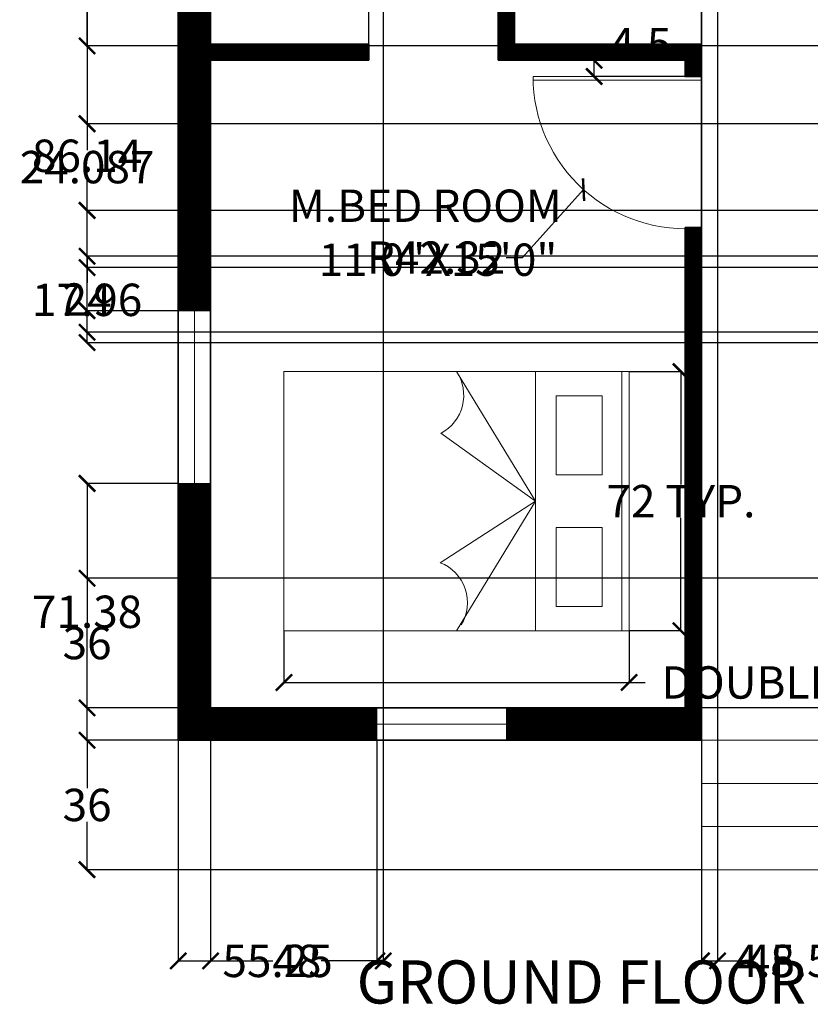
# Model space of a CAD drawing. Units: inches. Extents: x -1 to 426, y -6 to 532.
# Tile 1 of 4: x -1 to 219, y -6 to 267. Entities that reach past the tile are written whole.
import ezdxf

# ---------------------------------------------------------------- set-up
doc = ezdxf.new("R2010")
doc.units = ezdxf.units.IN
doc.header["$MEASUREMENT"] = 0
for name, color, linetype, lineweight in [('A-ANNO-DIMS', 2, 'Continuous', 18), ('A-ANNO-TEXT', 7, 'Continuous', 35), ('A-AREA-IDEN', 7, 'Continuous', 25), ('A-DOOR', 3, 'Continuous', 18), ('A-FLOR-STRS', 42, 'Continuous', 18), ('A-FURN', 8, 'Continuous', 18), ('A-GLAZ', 4, 'Continuous', 18)]:
    doc.layers.add(name, color=color, linetype=linetype, lineweight=lineweight)
doc.layers.add('A-WALL', color=159, linetype='Continuous', lineweight=35, true_color=0x223569)
doc.layers.add('A-WALL-PATT', color=177, linetype='Continuous', lineweight=13, true_color=0x2c4178)
doc.styles.get("Standard").update_dxf_attribs({"font": 'arial.ttf'})
doc.dimstyles.get("Standard").update_dxf_attribs({"dimtxt": 9, "dimasz": 4.5, "dimexe": 0.18, "dimexo": 0.0625, "dimgap": 0.09, "dimtad": 0, "dimtih": 1, "dimtoh": 1, "dimdec": 1, "dimzin": 0, "dimdsep": 46, "dimlunit": 4, "dimtxsty": 'Standard', "dimblk": 'ARCHTICK', "dimcen": 0.09, "dimadec": 0, "dimazin": 0, "dimtfac": 1, "dimtdec": 1, "dimtofl": 0, "dimtmove": 0, "dimatfit": 3, "dimfxl": 1, "dimtolj": 1, "dimtzin": 0, "dimarcsym": 0})

# ---------------------------------------------------------------- blocks, each defined once
blk = doc.blocks.new('WIN-36IN')
for p, q in [((0, 4.5), (36, 4.5)), ((0, -4.5), (0, 4.5)), ((36, 4.5), (36, -4.5)), ((0, 0), (36, 0)), ((36, -4.5), (0, -4.5))]:
    blk.add_line(p, q)
blk = doc.blocks.new('WIN-48IN')
for p, q in [((-4.5, 48), (4.5, 48)), ((-4.5, 0), (-4.5, 48)), ((0, 48), (0, 0)), ((4.5, 48), (4.5, 0)), ((4.5, 0), (-4.5, 0))]:
    blk.add_line(p, q)
blk = doc.blocks.new('BED-DOUBLE')
for p, q in [((-96, 0), (-96, 72)), ((-96, 72), (0, 72)), ((-26, 36), (-48, 72)), ((-26, 72), (-26, 0)), ((-2, 72), (-2, 0)), ((0, 72), (0, 0)), ((-52.33, 54.93), (-26, 36)), ((-26, 36), (-52.6, 18.9)), ((-48, 0), (-26, 36)), ((0, 0), (-96, 0))]:
    blk.add_line(p, q)
for points in [[(-7.5, 65.27), (-7.5, 43.28), (-20.33, 43.28), (-20.33, 65.27)], [(-7.5, 6.73), (-7.5, 28.72), (-20.33, 28.72), (-20.33, 6.73)]]:
    blk.add_lwpolyline(points, close=True)
for centre, start, end in [((-57.86, 65.42), 297.83, 33.7219), ((-56.81, 7.81), 328.371, 69.2037)]:
    blk.add_arc(centre, 11.86, start, end)
blk = doc.blocks.new('_ArchTick')
at = {"color": 0, "linetype": 'ByBlock', "const_width": 0.15}
blk.add_lwpolyline([(-0.5, -0.5), (0.5, 0.5)], dxfattribs=at)
blk = doc.blocks.new('*D11')
at = {"layer": 'A-ANNO-DIMS', "color": 0, "lineweight": -2, "transparency": 16777216}
for p, q in [((72.72, 97.36), (72.72, 82.85)), ((168.72, 97.36), (168.72, 82.85)), ((72.72, 83.03), (168.72, 83.03)), ((168.72, 83.03), (173.22, 83.03))]:
    blk.add_line(p, q, dxfattribs=at)
at = {"layer": 'Defpoints', "color": 0, "transparency": 16777216}
for p in [(72.72, 97.43), (168.72, 97.43), (168.72, 83.03)]:
    blk.add_point(p, dxfattribs=at)
at = {"layer": 'A-ANNO-DIMS', "color": 0, "lineweight": -2, "transparency": 16777216, "xscale": 4.5, "yscale": 4.5, "zscale": 4.5, "rotation": 180}
blk.add_blockref('_ArchTick', (72.72, 83.03), dxfattribs=at)
at = {"layer": 'A-ANNO-DIMS', "color": 0, "lineweight": -2, "transparency": 16777216, "xscale": 4.5, "yscale": 4.5, "zscale": 4.5}
blk.add_blockref('_ArchTick', (168.72, 83.03), dxfattribs=at)
at = {"layer": 'A-ANNO-DIMS', "color": 0, "transparency": 16777216, "insert": (237.26, 83.03), "char_height": 9, "attachment_point": 5}
blk.add_mtext('\\A1;DOUBLE BED 96 TYP.', dxfattribs=at)
blk = doc.blocks.new('*D12')
at = {"layer": 'A-ANNO-DIMS', "color": 0, "lineweight": -2, "transparency": 16777216}
for p, q in [((168.78, 169.43), (183.3, 169.43)), ((183.12, 169.43), (183.12, 138.04)), ((183.12, 97.43), (183.12, 128.81)), ((168.78, 97.43), (183.3, 97.43))]:
    blk.add_line(p, q, dxfattribs=at)
at = {"layer": 'Defpoints', "color": 0, "transparency": 16777216}
for p in [(168.72, 169.43), (183.12, 169.43), (168.72, 97.43)]:
    blk.add_point(p, dxfattribs=at)
at = {"layer": 'A-ANNO-DIMS', "color": 0, "lineweight": -2, "transparency": 16777216, "xscale": 4.5, "yscale": 4.5, "zscale": 4.5}
for p, rotation in [((183.12, 169.43), 90), ((183.12, 97.43), 270)]:
    blk.add_blockref('_ArchTick', p, dxfattribs=dict(at, rotation=rotation))
at = {"layer": 'A-ANNO-DIMS', "color": 0, "transparency": 16777216, "insert": (183.12, 133.43), "char_height": 9, "attachment_point": 5}
blk.add_mtext('\\A1;72 TYP.', dxfattribs=at)
blk = doc.blocks.new('*D19')
at = {"layer": 'A-ANNO-DIMS', "color": 0, "lineweight": -2, "transparency": 16777216}
for p, q in [((188.76, 66.98), (17.79, 66.98)), ((17.97, 66.98), (17.97, 53.67)), ((17.97, 30.98), (17.97, 44.29)), ((188.76, 30.98), (17.79, 30.98))]:
    blk.add_line(p, q, dxfattribs=at)
at = {"layer": 'Defpoints', "color": 0, "transparency": 16777216}
for p in [(17.97, 66.98), (188.82, 66.98), (188.82, 30.98)]:
    blk.add_point(p, dxfattribs=at)
at = {"layer": 'A-ANNO-DIMS', "color": 0, "lineweight": -2, "transparency": 16777216, "xscale": 4.5, "yscale": 4.5, "zscale": 4.5}
for p, rotation in [((17.97, 66.98), 90), ((17.97, 30.98), 270)]:
    blk.add_blockref('_ArchTick', p, dxfattribs=dict(at, rotation=rotation))
at = {"layer": 'A-ANNO-DIMS', "color": 0, "transparency": 16777216, "insert": (17.97, 48.98), "char_height": 9, "attachment_point": 5}
blk.add_mtext('\\A1;36', dxfattribs=at)
blk = doc.blocks.new('*D20')
at = {"layer": 'A-ANNO-DIMS', "color": 0, "lineweight": -2, "transparency": 16777216}
for p, q in [((43.32, 67.04), (43.32, 526.02)), ((43.32, 525.84), (101.19, 525.84)), ((188.82, 525.84), (130.96, 525.84)), ((188.82, 67.04), (188.82, 526.02))]:
    blk.add_line(p, q, dxfattribs=at)
at = {"layer": 'Defpoints', "color": 0, "transparency": 16777216}
for p in [(188.82, 525.84), (43.32, 66.98), (188.82, 66.98)]:
    blk.add_point(p, dxfattribs=at)
at = {"layer": 'A-ANNO-DIMS', "color": 0, "lineweight": -2, "transparency": 16777216, "xscale": 4.5, "yscale": 4.5, "zscale": 4.5, "rotation": 180}
blk.add_blockref('_ArchTick', (43.32, 525.84), dxfattribs=at)
at = {"layer": 'A-ANNO-DIMS', "color": 0, "lineweight": -2, "transparency": 16777216, "xscale": 4.5, "yscale": 4.5, "zscale": 4.5}
blk.add_blockref('_ArchTick', (188.82, 525.84), dxfattribs=at)
at = {"layer": 'A-ANNO-DIMS', "color": 0, "transparency": 16777216, "insert": (116.07, 525.84), "char_height": 9, "attachment_point": 5}
blk.add_mtext('\\A1;145.5', dxfattribs=at)
blk = doc.blocks.new('*D21')
at = {"layer": 'A-ANNO-DIMS', "color": 0, "lineweight": -2, "transparency": 16777216}
for p, q in [((188.82, 30.92), (188.82, 5.45)), ((237.32, 30.92), (237.32, 5.45)), ((188.82, 5.63), (201.08, 5.63)), ((237.32, 5.63), (225.07, 5.63))]:
    blk.add_line(p, q, dxfattribs=at)
at = {"layer": 'Defpoints', "color": 0, "transparency": 16777216}
for p in [(188.82, 30.98), (237.32, 30.98), (237.32, 5.63)]:
    blk.add_point(p, dxfattribs=at)
at = {"layer": 'A-ANNO-DIMS', "color": 0, "lineweight": -2, "transparency": 16777216, "xscale": 4.5, "yscale": 4.5, "zscale": 4.5, "rotation": 180}
blk.add_blockref('_ArchTick', (188.82, 5.63), dxfattribs=at)
at = {"layer": 'A-ANNO-DIMS', "color": 0, "lineweight": -2, "transparency": 16777216, "xscale": 4.5, "yscale": 4.5, "zscale": 4.5}
blk.add_blockref('_ArchTick', (237.32, 5.63), dxfattribs=at)
at = {"layer": 'A-ANNO-DIMS', "color": 0, "transparency": 16777216, "insert": (213.07, 5.63), "char_height": 9, "attachment_point": 5}
blk.add_mtext('\\A1;48.5', dxfattribs=at)
blk = doc.blocks.new('*D22')
at = {"layer": 'A-ANNO-DIMS', "color": 0, "lineweight": -2, "transparency": 16777216}
for p, q in [((52.32, 491.42), (52.32, 5.45)), ((100.32, 491.42), (100.32, 5.45)), ((52.32, 5.63), (69.6, 5.63)), ((100.32, 5.63), (83.05, 5.63))]:
    blk.add_line(p, q, dxfattribs=at)
at = {"layer": 'Defpoints', "color": 0, "transparency": 16777216}
for p in [(52.32, 491.48), (100.32, 491.48), (100.32, 5.63)]:
    blk.add_point(p, dxfattribs=at)
at = {"layer": 'A-ANNO-DIMS', "color": 0, "lineweight": -2, "transparency": 16777216, "xscale": 4.5, "yscale": 4.5, "zscale": 4.5, "rotation": 180}
blk.add_blockref('_ArchTick', (52.32, 5.63), dxfattribs=at)
at = {"layer": 'A-ANNO-DIMS', "color": 0, "lineweight": -2, "transparency": 16777216, "xscale": 4.5, "yscale": 4.5, "zscale": 4.5}
blk.add_blockref('_ArchTick', (100.32, 5.63), dxfattribs=at)
at = {"layer": 'A-ANNO-DIMS', "color": 0, "transparency": 16777216, "insert": (76.32, 5.63), "char_height": 9, "attachment_point": 5}
blk.add_mtext('\\A1;48', dxfattribs=at)
blk = doc.blocks.new('*D24')
at = {"layer": 'A-ANNO-DIMS', "color": 0, "lineweight": -2, "transparency": 16777216}
for p, q in [((43.32, 66.92), (43.32, 5.45)), ((98.58, 66.92), (98.58, 5.45)), ((43.32, 5.63), (55.64, 5.63)), ((98.58, 5.63), (86.26, 5.63))]:
    blk.add_line(p, q, dxfattribs=at)
at = {"layer": 'Defpoints', "color": 0, "transparency": 16777216}
for p in [(43.32, 66.98), (98.58, 66.98), (98.58, 5.63)]:
    blk.add_point(p, dxfattribs=at)
at = {"layer": 'A-ANNO-DIMS', "color": 0, "lineweight": -2, "transparency": 16777216, "xscale": 4.5, "yscale": 4.5, "zscale": 4.5, "rotation": 180}
blk.add_blockref('_ArchTick', (43.32, 5.63), dxfattribs=at)
at = {"layer": 'A-ANNO-DIMS', "color": 0, "lineweight": -2, "transparency": 16777216, "xscale": 4.5, "yscale": 4.5, "zscale": 4.5}
blk.add_blockref('_ArchTick', (98.58, 5.63), dxfattribs=at)
at = {"layer": 'A-ANNO-DIMS', "color": 0, "transparency": 16777216, "insert": (70.95, 5.63), "char_height": 9, "attachment_point": 5}
blk.add_mtext('\\A1;55.25', dxfattribs=at)
blk = doc.blocks.new('*D25')
at = {"layer": 'A-ANNO-DIMS', "color": 0, "lineweight": -2, "transparency": 16777216}
for p, q in [((43.26, 138.36), (17.79, 138.36)), ((17.97, 138.36), (17.97, 107.36)), ((17.97, 66.98), (17.97, 97.98)), ((43.26, 66.98), (17.79, 66.98))]:
    blk.add_line(p, q, dxfattribs=at)
at = {"layer": 'Defpoints', "color": 0, "transparency": 16777216}
for p in [(17.97, 138.36), (43.32, 138.36), (43.32, 66.98)]:
    blk.add_point(p, dxfattribs=at)
at = {"layer": 'A-ANNO-DIMS', "color": 0, "lineweight": -2, "transparency": 16777216, "xscale": 4.5, "yscale": 4.5, "zscale": 4.5}
for p, rotation in [((17.97, 138.36), 90), ((17.97, 66.98), 270)]:
    blk.add_blockref('_ArchTick', p, dxfattribs=dict(at, rotation=rotation))
at = {"layer": 'A-ANNO-DIMS', "color": 0, "transparency": 16777216, "insert": (17.97, 102.67), "char_height": 9, "attachment_point": 5}
blk.add_mtext('\\A1;71.38', dxfattribs=at)
blk = doc.blocks.new('*D26')
at = {"layer": 'A-ANNO-DIMS', "color": 0, "lineweight": -2, "transparency": 16777216}
for p, q in [((43.26, 272.5), (17.79, 272.5)), ((17.97, 272.5), (17.97, 234.11)), ((17.97, 186.36), (17.97, 224.74)), ((43.26, 186.36), (17.79, 186.36))]:
    blk.add_line(p, q, dxfattribs=at)
at = {"layer": 'Defpoints', "color": 0, "transparency": 16777216}
for p in [(17.97, 272.5), (43.32, 272.5), (43.32, 186.36)]:
    blk.add_point(p, dxfattribs=at)
at = {"layer": 'A-ANNO-DIMS', "color": 0, "lineweight": -2, "transparency": 16777216, "xscale": 4.5, "yscale": 4.5, "zscale": 4.5}
for p, rotation in [((17.97, 272.5), 90), ((17.97, 186.36), 270)]:
    blk.add_blockref('_ArchTick', p, dxfattribs=dict(at, rotation=rotation))
at = {"layer": 'A-ANNO-DIMS', "color": 0, "transparency": 16777216, "insert": (17.97, 229.43), "char_height": 9, "attachment_point": 5}
blk.add_mtext('\\A1;86.14', dxfattribs=at)
blk = doc.blocks.new('*D32')
at = {"layer": 'A-ANNO-DIMS', "color": 0, "lineweight": -2, "transparency": 16777216}
for p, q in [((331.76, 293.06), (17.79, 293.06)), ((17.97, 293.06), (17.97, 281.21)), ((17.97, 259.98), (17.97, 271.83)), ((331.76, 259.98), (17.79, 259.98))]:
    blk.add_line(p, q, dxfattribs=at)
at = {"layer": 'Defpoints', "color": 0, "transparency": 16777216}
for p in [(17.97, 293.06), (331.82, 293.06), (331.82, 259.98)]:
    blk.add_point(p, dxfattribs=at)
at = {"layer": 'A-ANNO-DIMS', "color": 0, "lineweight": -2, "transparency": 16777216, "xscale": 4.5, "yscale": 4.5, "zscale": 4.5}
for p, rotation in [((17.97, 293.06), 90), ((17.97, 259.98), 270)]:
    blk.add_blockref('_ArchTick', p, dxfattribs=dict(at, rotation=rotation))
at = {"layer": 'A-ANNO-DIMS', "color": 0, "transparency": 16777216, "insert": (17.97, 276.52), "char_height": 9, "attachment_point": 5}
blk.add_mtext('\\A1;33.08', dxfattribs=at)
blk = doc.blocks.new('*D34')
at = {"layer": 'A-ANNO-DIMS', "color": 0, "lineweight": -2, "transparency": 16777216}
for p, q in [((237.26, 111.98), (17.79, 111.98)), ((17.97, 111.98), (17.97, 98.67)), ((17.97, 75.98), (17.97, 89.29)), ((237.26, 75.98), (17.79, 75.98))]:
    blk.add_line(p, q, dxfattribs=at)
at = {"layer": 'Defpoints', "color": 0, "transparency": 16777216}
for p in [(17.97, 111.98), (237.32, 111.98), (237.32, 75.98)]:
    blk.add_point(p, dxfattribs=at)
at = {"layer": 'A-ANNO-DIMS', "color": 0, "lineweight": -2, "transparency": 16777216, "xscale": 4.5, "yscale": 4.5, "zscale": 4.5}
for p, rotation in [((17.97, 111.98), 90), ((17.97, 75.98), 270)]:
    blk.add_blockref('_ArchTick', p, dxfattribs=dict(at, rotation=rotation))
at = {"layer": 'A-ANNO-DIMS', "color": 0, "transparency": 16777216, "insert": (17.97, 93.98), "char_height": 9, "attachment_point": 5}
blk.add_mtext('\\A1;36', dxfattribs=at)
blk = doc.blocks.new('*D37')
at = {"layer": 'A-ANNO-DIMS', "color": 0, "lineweight": -2, "transparency": 16777216}
for p, q in [((258.34, 198.36), (17.79, 198.36)), ((17.97, 198.36), (17.97, 194.07)), ((17.97, 180.4), (17.97, 184.7)), ((258.34, 180.4), (17.79, 180.4))]:
    blk.add_line(p, q, dxfattribs=at)
at = {"layer": 'Defpoints', "color": 0, "transparency": 16777216}
for p in [(17.97, 198.36), (258.4, 198.36), (258.4, 180.4)]:
    blk.add_point(p, dxfattribs=at)
at = {"layer": 'A-ANNO-DIMS', "color": 0, "lineweight": -2, "transparency": 16777216, "xscale": 4.5, "yscale": 4.5, "zscale": 4.5}
for p, rotation in [((17.97, 198.36), 90), ((17.97, 180.4), 270)]:
    blk.add_blockref('_ArchTick', p, dxfattribs=dict(at, rotation=rotation))
at = {"layer": 'A-ANNO-DIMS', "color": 0, "transparency": 16777216, "insert": (17.97, 189.38), "char_height": 9, "attachment_point": 5}
blk.add_mtext('\\A1;17.96', dxfattribs=at)
blk = doc.blocks.new('*D39')
at = {"layer": 'A-ANNO-DIMS', "color": 0, "lineweight": -2, "transparency": 16777216}
for p, q in [((96.36, 256.04), (96.36, 526.02)), ((96.36, 525.84), (132.32, 525.84)), ((132.32, 256.04), (132.32, 526.02)), ((132.32, 525.84), (136.82, 525.84))]:
    blk.add_line(p, q, dxfattribs=at)
at = {"layer": 'Defpoints', "color": 0, "transparency": 16777216}
for p in [(132.32, 525.84), (96.36, 255.98), (132.32, 255.98)]:
    blk.add_point(p, dxfattribs=at)
at = {"layer": 'A-ANNO-DIMS', "color": 0, "lineweight": -2, "transparency": 16777216, "xscale": 4.5, "yscale": 4.5, "zscale": 4.5, "rotation": 180}
blk.add_blockref('_ArchTick', (96.36, 525.84), dxfattribs=at)
at = {"layer": 'A-ANNO-DIMS', "color": 0, "lineweight": -2, "transparency": 16777216, "xscale": 4.5, "yscale": 4.5, "zscale": 4.5}
blk.add_blockref('_ArchTick', (132.32, 525.84), dxfattribs=at)
at = {"layer": 'A-ANNO-DIMS', "color": 0, "transparency": 16777216, "insert": (155.63, 525.84), "char_height": 9, "attachment_point": 5}
blk.add_mtext('\\A1;35.965', dxfattribs=at)
blk = doc.blocks.new('*D45')
at = {"layer": 'A-ANNO-DIMS', "color": 0, "lineweight": -2, "transparency": 16777216}
for p, q in [((241.76, 201.48), (17.79, 201.48)), ((17.97, 201.48), (17.97, 194.09)), ((17.97, 177.48), (17.97, 184.87)), ((241.76, 177.48), (17.79, 177.48))]:
    blk.add_line(p, q, dxfattribs=at)
at = {"layer": 'Defpoints', "color": 0, "transparency": 16777216}
for p in [(17.97, 201.48), (241.82, 201.48), (241.82, 177.48)]:
    blk.add_point(p, dxfattribs=at)
at = {"layer": 'A-ANNO-DIMS', "color": 0, "lineweight": -2, "transparency": 16777216, "xscale": 4.5, "yscale": 4.5, "zscale": 4.5}
for p, rotation in [((17.97, 201.48), 90), ((17.97, 177.48), 270)]:
    blk.add_blockref('_ArchTick', p, dxfattribs=dict(at, rotation=rotation))
at = {"layer": 'A-ANNO-DIMS', "color": 0, "transparency": 16777216, "insert": (17.97, 189.48), "char_height": 9, "attachment_point": 5}
blk.add_mtext('\\A1;24', dxfattribs=at)
blk = doc.blocks.new('*D47')
at = {"layer": 'A-ANNO-DIMS', "color": 0, "lineweight": -2, "transparency": 16777216}
for p, q in [((188.82, 412.42), (188.82, 5.45)), ((193.32, 412.42), (193.32, 5.45)), ((188.82, 5.63), (193.32, 5.63)), ((193.32, 5.63), (197.82, 5.63))]:
    blk.add_line(p, q, dxfattribs=at)
at = {"layer": 'Defpoints', "color": 0, "transparency": 16777216}
for p in [(188.82, 412.48), (193.32, 412.48), (193.32, 5.63)]:
    blk.add_point(p, dxfattribs=at)
at = {"layer": 'A-ANNO-DIMS', "color": 0, "lineweight": -2, "transparency": 16777216, "xscale": 4.5, "yscale": 4.5, "zscale": 4.5, "rotation": 180}
blk.add_blockref('_ArchTick', (188.82, 5.63), dxfattribs=at)
at = {"layer": 'A-ANNO-DIMS', "color": 0, "lineweight": -2, "transparency": 16777216, "xscale": 4.5, "yscale": 4.5, "zscale": 4.5}
blk.add_blockref('_ArchTick', (193.32, 5.63), dxfattribs=at)
at = {"layer": 'A-ANNO-DIMS', "color": 0, "transparency": 16777216, "insert": (206.32, 5.63), "char_height": 9, "attachment_point": 5}
blk.add_mtext('\\A1;4.5', dxfattribs=at)
blk = doc.blocks.new('*D51')
at = {"layer": 'A-ANNO-DIMS', "color": 0, "lineweight": -2, "transparency": 16777216}
for p, q in [((158.97, 255.98), (158.97, 260.48)), ((158.97, 260.48), (163.47, 260.48)), ((184.26, 255.98), (158.79, 255.98)), ((158.97, 251.48), (158.97, 255.98)), ((184.26, 251.48), (158.79, 251.48))]:
    blk.add_line(p, q, dxfattribs=at)
at = {"layer": 'Defpoints', "color": 0, "transparency": 16777216}
for p in [(158.97, 255.98), (184.32, 255.98), (184.32, 251.48)]:
    blk.add_point(p, dxfattribs=at)
at = {"layer": 'A-ANNO-DIMS', "color": 0, "lineweight": -2, "transparency": 16777216, "xscale": 4.5, "yscale": 4.5, "zscale": 4.5}
for p, rotation in [((158.97, 255.98), 90), ((158.97, 251.48), 270)]:
    blk.add_blockref('_ArchTick', p, dxfattribs=dict(at, rotation=rotation))
at = {"layer": 'A-ANNO-DIMS', "color": 0, "transparency": 16777216, "insert": (171.96, 260.48), "char_height": 9, "attachment_point": 5}
blk.add_mtext('\\A1;4.5', dxfattribs=at)
blk = doc.blocks.new('*D53')
at = {"layer": 'A-ANNO-DIMS', "color": 0, "lineweight": -2, "transparency": 16777216}
for p, q in [((313, 238.33), (17.79, 238.33)), ((17.97, 238.33), (17.97, 230.97)), ((17.97, 214.24), (17.97, 221.6)), ((313, 214.24), (17.79, 214.24))]:
    blk.add_line(p, q, dxfattribs=at)
at = {"layer": 'Defpoints', "color": 0, "transparency": 16777216}
for p in [(17.97, 238.33), (313.06, 238.33), (313.06, 214.24)]:
    blk.add_point(p, dxfattribs=at)
at = {"layer": 'A-ANNO-DIMS', "color": 0, "lineweight": -2, "transparency": 16777216, "xscale": 4.5, "yscale": 4.5, "zscale": 4.5}
for p, rotation in [((17.97, 238.33), 90), ((17.97, 214.24), 270)]:
    blk.add_blockref('_ArchTick', p, dxfattribs=dict(at, rotation=rotation))
at = {"layer": 'A-ANNO-DIMS', "color": 0, "transparency": 16777216, "insert": (17.97, 226.28), "char_height": 9, "attachment_point": 5}
blk.add_mtext('\\A1;24.087', dxfattribs=at)
blk = doc.blocks.new('*D54')
at = {"layer": 'A-ANNO-DIMS', "color": 0, "lineweight": -2, "transparency": 16777216}
for p, q in [((184.23, 251.48), (184.41, 251.48)), ((184.32, 251.39), (184.32, 251.57)), ((139.06, 201.12), (156.04, 220.01)), ((134.56, 201.12), (139.06, 201.12))]:
    blk.add_line(p, q, dxfattribs=at)
at = {"layer": 'Defpoints', "color": 0, "transparency": 16777216}
for p in [(184.32, 251.48), (156.04, 220.01)]:
    blk.add_point(p, dxfattribs=at)
at = {"layer": 'A-ANNO-DIMS', "color": 0, "lineweight": -2, "transparency": 16777216, "xscale": 4.5, "yscale": 4.5, "zscale": 4.5, "rotation": 48.05222157853752}
blk.add_blockref('_ArchTick', (156.04, 220.01), dxfattribs=at)
at = {"layer": 'A-ANNO-DIMS', "color": 0, "transparency": 16777216, "insert": (115.03, 201.12), "char_height": 9, "attachment_point": 5}
blk.add_mtext('\\A1;R42.32', dxfattribs=at)

msp = doc.modelspace()

# ---------------------------------------------------------------- hatches: boundary and pattern name
at = {"layer": 'A-WALL-PATT'}
h = msp.add_hatch(dxfattribs=at)
h.set_pattern_fill('ANSI31', color=256)
h.set_pattern_definition([(45, (-574.8435, 0), (-0.088388348, 0.088388348), [])])
h.paths.add_polyline_path([(100.3238, 500.4824), (43.3238, 500.4824), (43.3238, 452.5693), (52.3238, 452.5693), (52.3238, 491.4824), (100.3238, 491.4824)])
h.paths.add_polyline_path([(242.3238, 500.4824), (136.3238, 500.4824), (136.3238, 491.4824), (184.3238, 491.4824), (184.3238, 407.9824), (188.8238, 407.9824), (193.3238, 407.9824), (193.3238, 412.4824), (188.8238, 412.4824), (188.8238, 491.4824), (242.3238, 491.4824)])
h.paths.add_polyline_path([(340.8238, 500.4824), (278.3238, 500.4824), (278.3238, 491.4824), (331.8238, 491.4824), (331.8238, 478.8941), (340.8238, 478.8941)])
h.paths.add_polyline_path([(331.8238, 412.4824), (229.3238, 412.4824), (229.3238, 407.9824), (331.8238, 407.9824)])
h.paths.add_polyline_path([(340.8238, 430.8941), (331.8238, 430.8941), (331.8238, 341.0593), (340.8238, 341.0593)])
h.paths.add_polyline_path([(340.8238, 293.0593), (331.8238, 293.0593), (331.8238, 259.9824), (282.3238, 259.9824), (282.3238, 255.4824), (331.8238, 255.4824), (331.8238, 237.2917), (340.8238, 237.2917)])
h.paths.add_polyline_path([(340.8238, 153.5275), (340.8238, 201.2917), (331.8238, 201.2917), (331.8238, 177.4824), (241.8238, 177.4824), (241.8238, 255.4824), (246.3238, 255.4824), (246.3238, 259.9824), (237.3238, 259.9824), (237.3238, 255.4824), (237.3238, 172.9824), (331.8238, 172.9824), (331.8238, 153.5275), (331.8238, 75.9824), (237.3238, 75.9824), (237.3238, 66.9824), (340.8238, 66.9824)])
h.paths.add_polyline_path([(98.5766, 75.9824), (52.3238, 75.9824), (52.3238, 138.3606), (43.3238, 138.3606), (43.3238, 66.9824), (52.3238, 66.9824), (98.5766, 66.9824)])
h.paths.add_polyline_path([(188.8238, 75.9824), (188.8238, 153.5275), (188.8238, 209.4042, -0.02664097), (184.3238, 209.1642), (184.3238, 153.5275), (184.3238, 75.9824), (136.8238, 75.9824), (134.5766, 75.9824), (134.5766, 66.9824), (136.8238, 66.9824), (188.8238, 66.9824)])
h.paths.add_polyline_path([(52.3238, 255.9824), (96.3583, 255.9824), (96.3583, 260.4824), (52.3238, 260.4824), (52.3238, 272.4986), (43.3238, 272.4986), (43.3238, 186.3606), (52.3238, 186.3606)])
h.paths.add_polyline_path([(52.3238, 404.5693), (43.3238, 404.5693), (43.3238, 349.9808), (52.3238, 349.9808), (52.3238, 360.9824), (184.3238, 360.9824), (184.3238, 312.9824), (173.036, 312.9824), (173.036, 308.4824), (184.3238, 308.4824), (188.8238, 308.4824), (188.8238, 365.4824), (184.3238, 365.4824), (52.3238, 365.4824)])
h.paths.add_polyline_path([(188.8238, 260.4824), (136.8238, 260.4824), (136.8238, 308.4824), (136.8238, 312.9824), (52.3238, 312.9824), (52.3238, 332.4824), (43.3238, 332.4824), (43.3238, 308.4824), (43.3238, 296.4986), (52.3238, 296.4986), (52.3238, 298.8674), (52.3238, 308.4824), (132.3238, 308.4824), (132.3238, 260.4824), (132.3238, 255.9824), (136.8238, 255.9824), (184.3238, 255.9824), (184.3238, 251.4824), (186.5738, 251.4824), (188.8238, 251.4824), (188.8238, 255.9824)])

# ---------------------------------------------------------------- linework, layer by layer
at = {"layer": 'A-DOOR'}
for p, q in [((186.5738, 251.4824), (142.0056, 251.4824)), ((186.5738, 250.4824), (142.0174, 250.4824)), ((184.3238, 250.4824), (188.8238, 250.4824)), ((188.8238, 251.4824), (188.8238, 209.4042))]:
    msp.add_line(p, q, dxfattribs=at)
msp.add_arc((184.3238, 251.4824), 42.3182, 180, 276.104216, dxfattribs=at)
at = {"layer": 'A-FLOR-STRS'}
for p, q in [((188.8238, 66.9824), (188.8238, 30.9824)), ((237.3238, 66.9824), (188.8238, 66.9824)), ((237.3238, 54.9824), (188.8238, 54.9824)), ((237.3238, 42.9824), (188.8238, 42.9824)), ((237.3238, 30.9824), (188.8238, 30.9824))]:
    msp.add_line(p, q, dxfattribs=at)
at = {"layer": 'A-WALL'}
for p, q in [((43.3238, 500.4824), (43.3238, 153.5275)), ((52.3238, 308.4824), (52.3238, 260.4824)), ((132.3238, 308.4824), (132.3238, 260.4824)), ((136.8238, 308.4824), (136.8238, 260.4824)), ((52.3238, 260.4824), (96.3583, 260.4824)), ((96.3583, 260.4824), (96.3583, 255.9824)), ((132.3238, 260.4824), (132.3238, 255.9824)), ((136.8238, 260.4824), (188.8238, 260.4824)), ((188.8238, 255.9824), (188.8238, 260.4824)), ((52.3238, 255.9824), (96.3583, 255.9824)), ((52.3238, 255.9824), (52.3238, 153.5275)), ((132.3238, 255.9824), (136.8238, 255.9824)), ((136.8238, 255.9824), (184.3238, 255.9824)), ((184.3238, 255.9824), (184.3238, 251.4824)), ((188.8238, 255.9824), (188.8238, 251.4824)), ((184.3238, 251.4824), (188.8238, 251.4824)), ((184.3238, 209.4824), (188.8238, 209.4824)), ((184.3238, 209.4824), (184.3238, 153.5275)), ((188.8238, 209.4824), (188.8238, 153.5275)), ((43.3238, 153.5275), (43.3238, 66.9824)), ((52.3238, 153.5275), (52.3238, 75.9824)), ((184.3238, 153.5275), (184.3238, 75.9824)), ((188.8238, 153.5275), (188.8238, 75.9824)), ((52.3238, 75.9824), (136.8238, 75.9824)), ((136.8238, 75.9824), (184.3238, 75.9824)), ((188.8238, 75.9824), (188.8238, 66.9824)), ((52.3238, 66.9824), (43.3238, 66.9824)), ((52.3238, 66.9824), (136.8238, 66.9824)), ((136.8238, 66.9824), (188.8238, 66.9824))]:
    msp.add_line(p, q, dxfattribs=at)

# ---------------------------------------------------------------- block references
at = {"layer": 'A-FURN'}
msp.add_blockref('BED-DOUBLE', (168.7206, 97.4252), dxfattribs=at)
at = {"layer": 'A-GLAZ'}
for name, p in [('WIN-48IN', (47.8238, 138.3606)), ('WIN-36IN', (98.5766, 71.4824))]:
    msp.add_blockref(name, p, dxfattribs=at)

# ---------------------------------------------------------------- texts
at = {"layer": 'A-ANNO-TEXT', "insert": (85.5965, 5.7797), "char_height": 12, "attachment_point": 1}
msp.add_mtext_dynamic_manual_height_columns('  GROUND FLOOR PLAN', width=229.541527, gutter_width=1, heights=[0], dxfattribs=at)
at = {"layer": 'A-AREA-IDEN', "insert": (74.1099, 220.0428), "char_height": 9, "attachment_point": 1}
msp.add_mtext_dynamic_manual_height_columns('M.BED ROOM\\P   11\'0"X15\'0"', width=229.541527, gutter_width=1, heights=[0], dxfattribs=at)

# ---------------------------------------------------------------- dimensions: what is measured, and where the dimension line sits
at = {"layer": 'A-ANNO-DIMS'}
for base, p1, p2, override, picture, middle in [((188.8238, 525.8389), (43.3238, 66.9824), (188.8238, 66.9824), {"dimdec": 1, "dimlfac": 1, "dimrnd": 0, "dimzin": 0, "dimdsep": 46, "dimlunit": 2}, '*D20', (116.0738, 525.8389)), ((132.32378, 525.83891), (96.35834, 255.98241), (132.32378, 255.98241), {"dimdec": 3, "dimlfac": 1, "dimrnd": 0, "dimzin": 0, "dimdsep": 46, "dimlunit": 2}, '*D39', (155.62592, 525.83891)), ((100.3238, 5.6259), (52.3238, 491.4824), (100.3238, 491.4824), {"dimdec": 0, "dimlfac": 1, "dimrnd": 0, "dimzin": 0, "dimdsep": 46, "dimlunit": 2}, '*D22', (76.3238, 5.6259)), ((193.3238, 5.6259), (188.8238, 412.4824), (193.3238, 412.4824), {"dimdec": 1, "dimlfac": 1, "dimrnd": 0, "dimzin": 0, "dimdsep": 46, "dimlunit": 2}, '*D47', (206.3214, 5.6259)), ((98.5766, 5.6259), (43.3238, 66.9824), (98.5766, 66.9824), {"dimdec": 2, "dimlfac": 1, "dimrnd": 0, "dimzin": 0, "dimdsep": 46, "dimlunit": 2}, '*D24', (70.9502, 5.6259)), ((237.3238, 5.6259), (188.8238, 30.9824), (237.3238, 30.9824), {"dimdec": 1, "dimlfac": 1, "dimrnd": 0, "dimzin": 0, "dimdsep": 46, "dimlunit": 2}, '*D21', (213.0738, 5.6259))]:
    dim = msp.add_linear_dim(base=base, p1=p1, p2=p2, dimstyle='Standard', override=override, dxfattribs=at)
    dim.commit()
    dim.dimension.update_dxf_attribs({"geometry": picture, "text_midpoint": middle})
for base, p1, p2, override, picture, middle in [((17.9673, 293.0593), (331.8238, 259.9824), (331.8238, 293.0593), {"dimdec": 2, "dimlfac": 1, "dimrnd": 0, "dimzin": 0, "dimdsep": 46, "dimlunit": 2}, '*D32', (17.9673, 276.5209)), ((17.9673, 272.4986), (43.3238, 186.3606), (43.3238, 272.4986), {"dimdec": 2, "dimlfac": 1, "dimrnd": 0, "dimzin": 0, "dimdsep": 46, "dimlunit": 2}, '*D26', (17.9673, 229.4296)), ((158.9673, 255.9824), (184.3238, 251.4824), (184.3238, 255.9824), {"dimdec": 1, "dimlfac": 1, "dimrnd": 0, "dimzin": 0, "dimdsep": 46, "dimlunit": 2}, '*D51', (171.9649, 260.4824)), ((17.9673, 238.326), (313.0636, 214.2386), (313.0636, 238.326), {"dimdec": 3, "dimlfac": 1, "dimrnd": 0, "dimzin": 0, "dimdsep": 46, "dimlunit": 2}, '*D53', (17.9673, 226.2823)), ((17.9673, 201.4824), (241.8238, 177.4824), (241.8238, 201.4824), {"dimdec": 0, "dimlfac": 1, "dimrnd": 0, "dimzin": 0, "dimdsep": 46, "dimlunit": 2}, '*D45', (17.9673, 189.4824)), ((17.9673, 198.3607), (258.4022, 180.4022), (258.4022, 198.3607), {"dimdec": 2, "dimlfac": 1, "dimrnd": 0, "dimzin": 0, "dimdsep": 46, "dimlunit": 2}, '*D37', (17.9673, 189.3814)), ((17.9673, 138.3606), (43.3238, 66.9824), (43.3238, 138.3606), {"dimdec": 2, "dimlfac": 1, "dimrnd": 0, "dimzin": 0, "dimdsep": 46, "dimlunit": 2}, '*D25', (17.9673, 102.6715)), ((17.9673, 111.9824), (237.3238, 75.9824), (237.3238, 111.9824), {"dimdec": 0, "dimlfac": 1, "dimrnd": 0, "dimzin": 0, "dimdsep": 46, "dimlunit": 2}, '*D34', (17.9673, 93.9824)), ((17.9673, 66.9824), (188.8238, 30.9824), (188.8238, 66.9824), {"dimdec": 0, "dimlfac": 1, "dimrnd": 0, "dimzin": 0, "dimdsep": 46, "dimlunit": 2}, '*D19', (17.9673, 48.9824))]:
    dim = msp.add_linear_dim(base=base, p1=p1, p2=p2, angle=90, dimstyle='Standard', override=override, dxfattribs=at)
    dim.commit()
    dim.dimension.update_dxf_attribs({"geometry": picture, "text_midpoint": middle})
dim = msp.add_radius_dim(center=(184.3238, 251.4824), mpoint=(156.0361, 220.0081), dimstyle='Standard', override={"dimdec": 2, "dimlfac": 1, "dimrnd": 0, "dimzin": 0, "dimdsep": 46, "dimlunit": 2}, dxfattribs=at)
dim.commit()
dim.dimension.update_dxf_attribs({"geometry": '*D54', "text_midpoint": (115.0277, 201.1235), "dimtype": 164})
dim = msp.add_linear_dim(base=(183.1206, 169.4252), p1=(168.7206, 97.4252), p2=(168.7206, 169.4252), angle=90, text='<> TYP.', dimstyle='Standard', override={"dimdec": 0, "dimlfac": 1, "dimrnd": 0, "dimzin": 0, "dimdsep": 46, "dimlunit": 2}, dxfattribs=at)
dim.commit()
dim.dimension.update_dxf_attribs({"geometry": '*D12', "text_midpoint": (183.1206, 133.4252)})
dim = msp.add_linear_dim(base=(168.7206, 83.0252), p1=(72.7206, 97.4252), p2=(168.7206, 97.4252), text='DOUBLE BED <> TYP.', dimstyle='Standard', override={"dimdec": 0, "dimlfac": 1, "dimrnd": 0, "dimzin": 0, "dimdsep": 46, "dimlunit": 2}, dxfattribs=at)
dim.commit()
dim.dimension.update_dxf_attribs({"geometry": '*D11', "text_midpoint": (237.2622, 83.0252)})

doc.saveas('drawing.dxf')
